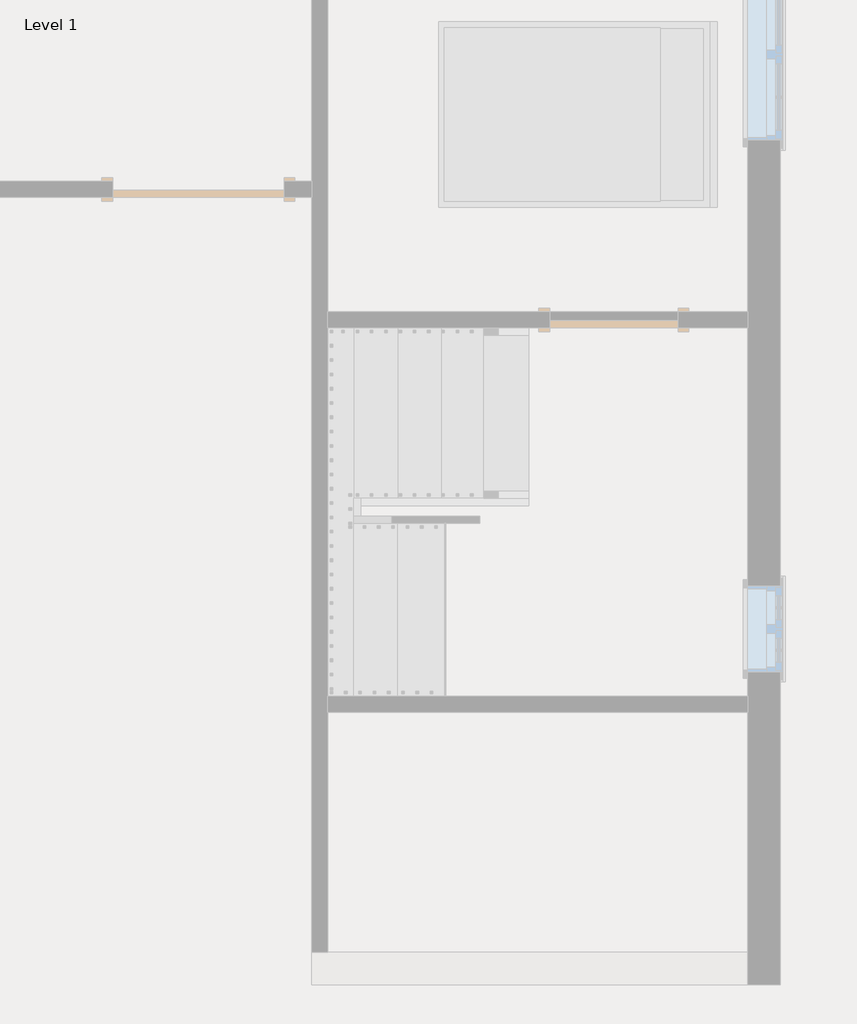
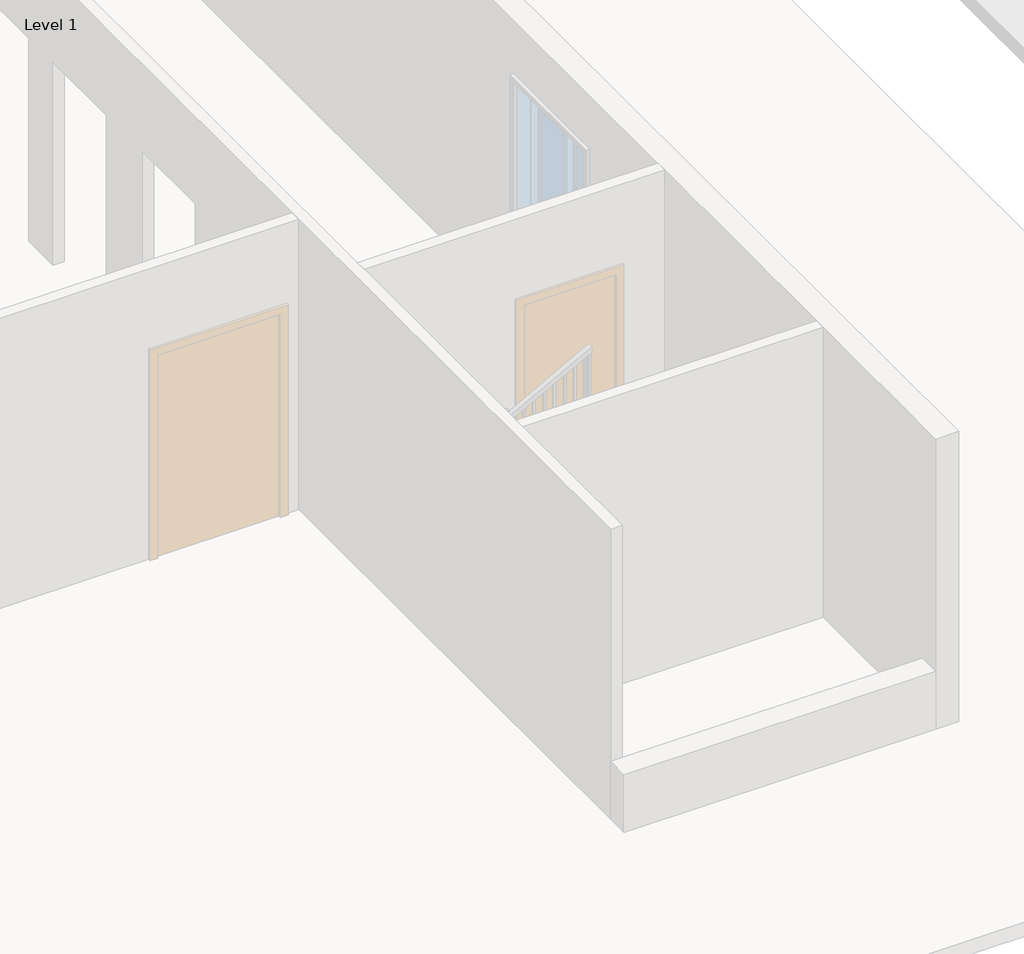
# One storey, part 3 of 7: 2 railings.
"""IFC4 building model written with IfcOpenShell, lengths in millimetres."""

from ifc_helpers import new_model, si_unit, frame, origin, place, context, project, spatial, polyline, outline, extrude, faceted_brep, element, save

model = new_model("IFC4")

# Units and contexts
model_context = context("Model", 3, world=origin())
ifc_project = project(units=[si_unit("LENGTHUNIT", "METRE", prefix="MILLI")], contexts=[model_context])

# Site, building, storey
site = spatial("IfcSite", under=ifc_project)
building = spatial("IfcBuilding", under=site)
storey = spatial("IfcBuildingStorey", under=building, Name="Level 1", Elevation=0.0)

# Railings
placement = place(None, origin())
element("IfcRailing", 1, ObjectType="Handrail - Rectangular", at=placement, inside=storey, context=model_context, shape_type="SolidModel", body=[
    faceted_brep([(7105.1820958, 5435.6, 1083.7333333), (7105.1820958, 5435.6, 1025.8977421), (7105.1820958, 5486.4, 1025.8977421), (7105.1820958, 5486.4, 1083.7333333), (5860.5820958, 5435.6, 1761.0666667), (5847.654197, 5435.6, 1710.2666667), (5847.654197, 5486.4, 1710.2666667), (5860.5820958, 5486.4, 1761.0666667), (5727.7, 5435.6, 1761.0666667), (5727.7, 5435.6, 1710.2666667), (5676.9, 5486.4, 1710.2666667), (5676.9, 5486.4, 1761.0666667), (5727.7, 2997.2, 1761.0666667), (5727.7, 2946.4, 1710.2666667), (5676.9, 2946.4, 1710.2666667), (5676.9, 2997.2, 1761.0666667), (5727.7, 2997.2, 1899.5526009), (5727.7, 2946.4, 1848.7526009), (5676.9, 2946.4, 1848.7526009), (5676.9, 2997.2, 1899.5526009), (5727.7, 2921.0, 1899.5526009), (5727.7, 2921.0, 1848.7526009), (5676.9, 2870.2, 1848.7526009), (5676.9, 2870.2, 1899.5526009), (5803.9, 2921.0, 1899.5526009), (5816.8278988, 2921.0, 1848.7526009), (5816.8278988, 2870.2, 1848.7526009), (5803.9, 2870.2, 1899.5526009), (7105.1820958, 2921.0, 2607.7333333), (7105.1820958, 2870.2, 2607.7333333), (7105.1820958, 2870.2, 2549.8977421), (7105.1820958, 2921.0, 2549.8977421)], [[[0, 1, 2, 3]], [[1, 0, 4, 5]], [[2, 1, 5, 6]], [[3, 2, 6, 7]], [[0, 3, 7, 4]], [[5, 4, 8, 9]], [[6, 5, 9, 10]], [[7, 6, 10, 11]], [[4, 7, 11, 8]], [[9, 8, 12, 13]], [[10, 9, 13, 14]], [[11, 10, 14, 15]], [[8, 11, 15, 12]], [[13, 12, 16, 17]], [[14, 13, 17, 18]], [[15, 14, 18, 19]], [[12, 15, 19, 16]], [[17, 16, 20, 21]], [[18, 17, 21, 22]], [[19, 18, 22, 23]], [[16, 19, 23, 20]], [[21, 20, 24, 25]], [[22, 21, 25, 26]], [[23, 22, 26, 27]], [[20, 23, 27, 24]], [[28, 29, 30, 31]], [[25, 24, 28, 31]], [[26, 25, 31, 30]], [[27, 26, 30, 29]], [[24, 27, 29, 28]]]),
    extrude(outline(polyline([(2510.4108873, 7032.625), (2500.0435403, 7013.575), (1524.0, 7013.575), (1524.0, 7032.625), (2510.4108873, 7032.625)])), frame((0.0, 2886.075, 0.0), z_axis=(0.0, 1.0, 0.0), x_axis=(0.0, 0.0, 1.0)), (0.0, 0.0, 1.0), 19.05),
    extrude(outline(polyline([(2455.1183703, 6931.025), (2444.7510233, 6911.975), (1524.0, 6911.975), (1524.0, 6931.025), (2455.1183703, 6931.025)])), frame((0.0, 2886.075, 0.0), z_axis=(0.0, 1.0, 0.0), x_axis=(0.0, 0.0, 1.0)), (0.0, 0.0, 1.0), 19.05),
    extrude(outline(polyline([(2399.8258533, 6829.425), (2389.4585063, 6810.375), (1524.0, 6810.375), (1524.0, 6829.425), (2399.8258533, 6829.425)])), frame((0.0, 2886.075, 0.0), z_axis=(0.0, 1.0, 0.0), x_axis=(0.0, 0.0, 1.0)), (0.0, 0.0, 1.0), 19.05),
    extrude(outline(polyline([(2344.5333363, 6727.825), (2334.1659893, 6708.775), (1354.6666667, 6708.775), (1354.6666667, 6727.825), (2344.5333363, 6727.825)])), frame((0.0, 2886.075, 0.0), z_axis=(0.0, 1.0, 0.0), x_axis=(0.0, 0.0, 1.0)), (0.0, 0.0, 1.0), 19.05),
    extrude(outline(polyline([(2289.2408192, 6626.225), (2278.8734723, 6607.175), (1354.6666667, 6607.175), (1354.6666667, 6626.225), (2289.2408192, 6626.225)])), frame((0.0, 2886.075, 0.0), z_axis=(0.0, 1.0, 0.0), x_axis=(0.0, 0.0, 1.0)), (0.0, 0.0, 1.0), 19.05),
    extrude(outline(polyline([(2233.9483022, 6524.625), (2223.5809553, 6505.575), (1354.6666667, 6505.575), (1354.6666667, 6524.625), (2233.9483022, 6524.625)])), frame((0.0, 2886.075, 0.0), z_axis=(0.0, 1.0, 0.0), x_axis=(0.0, 0.0, 1.0)), (0.0, 0.0, 1.0), 19.05),
    extrude(outline(polyline([(2178.6557852, 6423.025), (2168.2884383, 6403.975), (1185.3333333, 6403.975), (1185.3333333, 6423.025), (2178.6557852, 6423.025)])), frame((0.0, 2886.075, 0.0), z_axis=(0.0, 1.0, 0.0), x_axis=(0.0, 0.0, 1.0)), (0.0, 0.0, 1.0), 19.05),
    extrude(outline(polyline([(2123.3632682, 6321.425), (2112.9959213, 6302.375), (1185.3333333, 6302.375), (1185.3333333, 6321.425), (2123.3632682, 6321.425)])), frame((0.0, 2886.075, 0.0), z_axis=(0.0, 1.0, 0.0), x_axis=(0.0, 0.0, 1.0)), (0.0, 0.0, 1.0), 19.05),
    extrude(outline(polyline([(2068.0707512, 6219.825), (2057.7034043, 6200.775), (1185.3333333, 6200.775), (1185.3333333, 6219.825), (2068.0707512, 6219.825)])), frame((0.0, 2886.075, 0.0), z_axis=(0.0, 1.0, 0.0), x_axis=(0.0, 0.0, 1.0)), (0.0, 0.0, 1.0), 19.05),
    extrude(outline(polyline([(2012.7782342, 6118.225), (2002.4108873, 6099.175), (1016.0, 6099.175), (1016.0, 6118.225), (2012.7782342, 6118.225)])), frame((0.0, 2886.075, 0.0), z_axis=(0.0, 1.0, 0.0), x_axis=(0.0, 0.0, 1.0)), (0.0, 0.0, 1.0), 19.05),
    extrude(outline(polyline([(1957.4857172, 6016.625), (1947.1183703, 5997.575), (1016.0, 5997.575), (1016.0, 6016.625), (1957.4857172, 6016.625)])), frame((0.0, 2886.075, 0.0), z_axis=(0.0, 1.0, 0.0), x_axis=(0.0, 0.0, 1.0)), (0.0, 0.0, 1.0), 19.05),
    extrude(outline(polyline([(1902.1932002, 5915.025), (1891.8258533, 5895.975), (1016.0, 5895.975), (1016.0, 5915.025), (1902.1932002, 5915.025)])), frame((0.0, 2886.075, 0.0), z_axis=(0.0, 1.0, 0.0), x_axis=(0.0, 0.0, 1.0)), (0.0, 0.0, 1.0), 19.05),
    extrude(outline(polyline([(1846.9006832, 5813.425), (1836.5333363, 5794.375), (846.6666667, 5794.375), (846.6666667, 5813.425), (1846.9006832, 5813.425)])), frame((0.0, 2886.075, 0.0), z_axis=(0.0, 1.0, 0.0), x_axis=(0.0, 0.0, 1.0)), (0.0, 0.0, 1.0), 19.05),
    extrude(outline(polyline([(5692.775, 2930.525), (5711.825, 2930.525), (5711.825, 2911.475), (5692.775, 2911.475), (5692.775, 2930.525)])), frame((0.0, 0.0, 846.6666667), z_axis=(0.0, 0.0, 1.0), x_axis=(1.0, 0.0, 0.0)), (0.0, 0.0, 1.0), 1002.0859343),
    extrude(outline(polyline([(5692.775, 3032.125), (5711.825, 3032.125), (5711.825, 3013.075), (5692.775, 3013.075), (5692.775, 3032.125)])), frame((0.0, 0.0, 846.6666667), z_axis=(0.0, 0.0, 1.0), x_axis=(1.0, 0.0, 0.0)), (0.0, 0.0, 1.0), 863.6),
    extrude(outline(polyline([(5692.775, 3133.725), (5711.825, 3133.725), (5711.825, 3114.675), (5692.775, 3114.675), (5692.775, 3133.725)])), frame((0.0, 0.0, 846.6666667), z_axis=(0.0, 0.0, 1.0), x_axis=(1.0, 0.0, 0.0)), (0.0, 0.0, 1.0), 863.6),
    extrude(outline(polyline([(5692.775, 3235.325), (5711.825, 3235.325), (5711.825, 3216.275), (5692.775, 3216.275), (5692.775, 3235.325)])), frame((0.0, 0.0, 846.6666667), z_axis=(0.0, 0.0, 1.0), x_axis=(1.0, 0.0, 0.0)), (0.0, 0.0, 1.0), 863.6),
    extrude(outline(polyline([(5692.775, 3336.925), (5711.825, 3336.925), (5711.825, 3317.875), (5692.775, 3317.875), (5692.775, 3336.925)])), frame((0.0, 0.0, 846.6666667), z_axis=(0.0, 0.0, 1.0), x_axis=(1.0, 0.0, 0.0)), (0.0, 0.0, 1.0), 863.6),
    extrude(outline(polyline([(5692.775, 3438.525), (5711.825, 3438.525), (5711.825, 3419.475), (5692.775, 3419.475), (5692.775, 3438.525)])), frame((0.0, 0.0, 846.6666667), z_axis=(0.0, 0.0, 1.0), x_axis=(1.0, 0.0, 0.0)), (0.0, 0.0, 1.0), 863.6),
    extrude(outline(polyline([(5692.775, 3540.125), (5711.825, 3540.125), (5711.825, 3521.075), (5692.775, 3521.075), (5692.775, 3540.125)])), frame((0.0, 0.0, 846.6666667), z_axis=(0.0, 0.0, 1.0), x_axis=(1.0, 0.0, 0.0)), (0.0, 0.0, 1.0), 863.6),
    extrude(outline(polyline([(5692.775, 3641.725), (5711.825, 3641.725), (5711.825, 3622.675), (5692.775, 3622.675), (5692.775, 3641.725)])), frame((0.0, 0.0, 846.6666667), z_axis=(0.0, 0.0, 1.0), x_axis=(1.0, 0.0, 0.0)), (0.0, 0.0, 1.0), 863.6),
    extrude(outline(polyline([(5692.775, 3743.325), (5711.825, 3743.325), (5711.825, 3724.275), (5692.775, 3724.275), (5692.775, 3743.325)])), frame((0.0, 0.0, 846.6666667), z_axis=(0.0, 0.0, 1.0), x_axis=(1.0, 0.0, 0.0)), (0.0, 0.0, 1.0), 863.6),
    extrude(outline(polyline([(5692.775, 3844.925), (5711.825, 3844.925), (5711.825, 3825.875), (5692.775, 3825.875), (5692.775, 3844.925)])), frame((0.0, 0.0, 846.6666667), z_axis=(0.0, 0.0, 1.0), x_axis=(1.0, 0.0, 0.0)), (0.0, 0.0, 1.0), 863.6),
    extrude(outline(polyline([(5692.775, 3946.525), (5711.825, 3946.525), (5711.825, 3927.475), (5692.775, 3927.475), (5692.775, 3946.525)])), frame((0.0, 0.0, 846.6666667), z_axis=(0.0, 0.0, 1.0), x_axis=(1.0, 0.0, 0.0)), (0.0, 0.0, 1.0), 863.6),
    extrude(outline(polyline([(5692.775, 4048.125), (5711.825, 4048.125), (5711.825, 4029.075), (5692.775, 4029.075), (5692.775, 4048.125)])), frame((0.0, 0.0, 846.6666667), z_axis=(0.0, 0.0, 1.0), x_axis=(1.0, 0.0, 0.0)), (0.0, 0.0, 1.0), 863.6),
    extrude(outline(polyline([(5692.775, 4149.725), (5711.825, 4149.725), (5711.825, 4130.675), (5692.775, 4130.675), (5692.775, 4149.725)])), frame((0.0, 0.0, 846.6666667), z_axis=(0.0, 0.0, 1.0), x_axis=(1.0, 0.0, 0.0)), (0.0, 0.0, 1.0), 863.6),
    extrude(outline(polyline([(5692.775, 4251.325), (5711.825, 4251.325), (5711.825, 4232.275), (5692.775, 4232.275), (5692.775, 4251.325)])), frame((0.0, 0.0, 846.6666667), z_axis=(0.0, 0.0, 1.0), x_axis=(1.0, 0.0, 0.0)), (0.0, 0.0, 1.0), 863.6),
    extrude(outline(polyline([(5692.775, 4352.925), (5711.825, 4352.925), (5711.825, 4333.875), (5692.775, 4333.875), (5692.775, 4352.925)])), frame((0.0, 0.0, 846.6666667), z_axis=(0.0, 0.0, 1.0), x_axis=(1.0, 0.0, 0.0)), (0.0, 0.0, 1.0), 863.6),
    extrude(outline(polyline([(5692.775, 4454.525), (5711.825, 4454.525), (5711.825, 4435.475), (5692.775, 4435.475), (5692.775, 4454.525)])), frame((0.0, 0.0, 846.6666667), z_axis=(0.0, 0.0, 1.0), x_axis=(1.0, 0.0, 0.0)), (0.0, 0.0, 1.0), 863.6),
    extrude(outline(polyline([(5692.775, 4556.125), (5711.825, 4556.125), (5711.825, 4537.075), (5692.775, 4537.075), (5692.775, 4556.125)])), frame((0.0, 0.0, 846.6666667), z_axis=(0.0, 0.0, 1.0), x_axis=(1.0, 0.0, 0.0)), (0.0, 0.0, 1.0), 863.6),
    extrude(outline(polyline([(5692.775, 4657.725), (5711.825, 4657.725), (5711.825, 4638.675), (5692.775, 4638.675), (5692.775, 4657.725)])), frame((0.0, 0.0, 846.6666667), z_axis=(0.0, 0.0, 1.0), x_axis=(1.0, 0.0, 0.0)), (0.0, 0.0, 1.0), 863.6),
    extrude(outline(polyline([(5692.775, 4759.325), (5711.825, 4759.325), (5711.825, 4740.275), (5692.775, 4740.275), (5692.775, 4759.325)])), frame((0.0, 0.0, 846.6666667), z_axis=(0.0, 0.0, 1.0), x_axis=(1.0, 0.0, 0.0)), (0.0, 0.0, 1.0), 863.6),
    extrude(outline(polyline([(5692.775, 4860.925), (5711.825, 4860.925), (5711.825, 4841.875), (5692.775, 4841.875), (5692.775, 4860.925)])), frame((0.0, 0.0, 846.6666667), z_axis=(0.0, 0.0, 1.0), x_axis=(1.0, 0.0, 0.0)), (0.0, 0.0, 1.0), 863.6),
    extrude(outline(polyline([(5692.775, 4962.525), (5711.825, 4962.525), (5711.825, 4943.475), (5692.775, 4943.475), (5692.775, 4962.525)])), frame((0.0, 0.0, 846.6666667), z_axis=(0.0, 0.0, 1.0), x_axis=(1.0, 0.0, 0.0)), (0.0, 0.0, 1.0), 863.6),
    extrude(outline(polyline([(5692.775, 5064.125), (5711.825, 5064.125), (5711.825, 5045.075), (5692.775, 5045.075), (5692.775, 5064.125)])), frame((0.0, 0.0, 846.6666667), z_axis=(0.0, 0.0, 1.0), x_axis=(1.0, 0.0, 0.0)), (0.0, 0.0, 1.0), 863.6),
    extrude(outline(polyline([(5692.775, 5165.725), (5711.825, 5165.725), (5711.825, 5146.675), (5692.775, 5146.675), (5692.775, 5165.725)])), frame((0.0, 0.0, 846.6666667), z_axis=(0.0, 0.0, 1.0), x_axis=(1.0, 0.0, 0.0)), (0.0, 0.0, 1.0), 863.6),
    extrude(outline(polyline([(5692.775, 5267.325), (5711.825, 5267.325), (5711.825, 5248.275), (5692.775, 5248.275), (5692.775, 5267.325)])), frame((0.0, 0.0, 846.6666667), z_axis=(0.0, 0.0, 1.0), x_axis=(1.0, 0.0, 0.0)), (0.0, 0.0, 1.0), 863.6),
    extrude(outline(polyline([(5692.775, 5368.925), (5711.825, 5368.925), (5711.825, 5349.875), (5692.775, 5349.875), (5692.775, 5368.925)])), frame((0.0, 0.0, 846.6666667), z_axis=(0.0, 0.0, 1.0), x_axis=(1.0, 0.0, 0.0)), (0.0, 0.0, 1.0), 863.6),
    extrude(outline(polyline([(5793.9070958, 5470.525), (5793.9070958, 5451.475), (5774.8570958, 5451.475), (5774.8570958, 5470.525), (5793.9070958, 5470.525)])), frame((0.0, 0.0, 846.6666667), z_axis=(0.0, 0.0, 1.0), x_axis=(1.0, 0.0, 0.0)), (0.0, 0.0, 1.0), 863.6),
    extrude(outline(polyline([(1684.2242727, 5895.5070958), (1694.5916197, 5876.4570958), (677.3333333, 5876.4570958), (677.3333333, 5895.5070958), (1684.2242727, 5895.5070958)])), frame((0.0, 5451.475, 0.0), z_axis=(0.0, 1.0, 0.0), x_axis=(0.0, 0.0, 1.0)), (0.0, 0.0, 1.0), 19.05),
    extrude(outline(polyline([(1628.9317557, 5997.1070958), (1639.2991027, 5978.0570958), (677.3333333, 5978.0570958), (677.3333333, 5997.1070958), (1628.9317557, 5997.1070958)])), frame((0.0, 5451.475, 0.0), z_axis=(0.0, 1.0, 0.0), x_axis=(0.0, 0.0, 1.0)), (0.0, 0.0, 1.0), 19.05),
    extrude(outline(polyline([(1573.6392387, 6098.7070958), (1584.0065857, 6079.6570958), (677.3333333, 6079.6570958), (677.3333333, 6098.7070958), (1573.6392387, 6098.7070958)])), frame((0.0, 5451.475, 0.0), z_axis=(0.0, 1.0, 0.0), x_axis=(0.0, 0.0, 1.0)), (0.0, 0.0, 1.0), 19.05),
    extrude(outline(polyline([(1518.3467217, 6200.3070958), (1528.7140687, 6181.2570958), (508.0, 6181.2570958), (508.0, 6200.3070958), (1518.3467217, 6200.3070958)])), frame((0.0, 5451.475, 0.0), z_axis=(0.0, 1.0, 0.0), x_axis=(0.0, 0.0, 1.0)), (0.0, 0.0, 1.0), 19.05),
    extrude(outline(polyline([(1463.0542047, 6301.9070958), (1473.4215517, 6282.8570958), (508.0, 6282.8570958), (508.0, 6301.9070958), (1463.0542047, 6301.9070958)])), frame((0.0, 5451.475, 0.0), z_axis=(0.0, 1.0, 0.0), x_axis=(0.0, 0.0, 1.0)), (0.0, 0.0, 1.0), 19.05),
    extrude(outline(polyline([(1407.7616877, 6403.5070958), (1418.1290347, 6384.4570958), (508.0, 6384.4570958), (508.0, 6403.5070958), (1407.7616877, 6403.5070958)])), frame((0.0, 5451.475, 0.0), z_axis=(0.0, 1.0, 0.0), x_axis=(0.0, 0.0, 1.0)), (0.0, 0.0, 1.0), 19.05),
    extrude(outline(polyline([(1352.4691707, 6505.1070958), (1362.8365176, 6486.0570958), (338.6666667, 6486.0570958), (338.6666667, 6505.1070958), (1352.4691707, 6505.1070958)])), frame((0.0, 5451.475, 0.0), z_axis=(0.0, 1.0, 0.0), x_axis=(0.0, 0.0, 1.0)), (0.0, 0.0, 1.0), 19.05),
    extrude(outline(polyline([(1297.1766537, 6606.7070958), (1307.5440006, 6587.6570958), (338.6666667, 6587.6570958), (338.6666667, 6606.7070958), (1297.1766537, 6606.7070958)])), frame((0.0, 5451.475, 0.0), z_axis=(0.0, 1.0, 0.0), x_axis=(0.0, 0.0, 1.0)), (0.0, 0.0, 1.0), 19.05),
    extrude(outline(polyline([(1241.8841367, 6708.3070958), (1252.2514836, 6689.2570958), (338.6666667, 6689.2570958), (338.6666667, 6708.3070958), (1241.8841367, 6708.3070958)])), frame((0.0, 5451.475, 0.0), z_axis=(0.0, 1.0, 0.0), x_axis=(0.0, 0.0, 1.0)), (0.0, 0.0, 1.0), 19.05),
    extrude(outline(polyline([(1186.5916197, 6809.9070958), (1196.9589666, 6790.8570958), (169.3333333, 6790.8570958), (169.3333333, 6809.9070958), (1186.5916197, 6809.9070958)])), frame((0.0, 5451.475, 0.0), z_axis=(0.0, 1.0, 0.0), x_axis=(0.0, 0.0, 1.0)), (0.0, 0.0, 1.0), 19.05),
    extrude(outline(polyline([(1131.2991027, 6911.5070958), (1141.6664496, 6892.4570958), (169.3333333, 6892.4570958), (169.3333333, 6911.5070958), (1131.2991027, 6911.5070958)])), frame((0.0, 5451.475, 0.0), z_axis=(0.0, 1.0, 0.0), x_axis=(0.0, 0.0, 1.0)), (0.0, 0.0, 1.0), 19.05),
    extrude(outline(polyline([(1076.0065857, 7013.1070958), (1086.3739326, 6994.0570958), (169.3333333, 6994.0570958), (169.3333333, 7013.1070958), (1076.0065857, 7013.1070958)])), frame((0.0, 5451.475, 0.0), z_axis=(0.0, 1.0, 0.0), x_axis=(0.0, 0.0, 1.0)), (0.0, 0.0, 1.0), 19.05),
    extrude(outline(polyline([(5692.775, 2905.125), (5711.825, 2905.125), (5711.825, 2886.075), (5692.775, 2886.075), (5692.775, 2905.125)])), frame((0.0, 0.0, 846.6666667), z_axis=(0.0, 0.0, 1.0), x_axis=(1.0, 0.0, 0.0)), (0.0, 0.0, 1.0), 1002.0859343),
    extrude(outline(polyline([(5711.825, 5470.525), (5711.825, 5451.475), (5692.775, 5451.475), (5692.775, 5470.525), (5711.825, 5470.525)])), frame((0.0, 0.0, 846.6666667), z_axis=(0.0, 0.0, 1.0), x_axis=(1.0, 0.0, 0.0)), (0.0, 0.0, 1.0), 863.6),
    extrude(outline(polyline([(2549.8977421, 7105.1820958), (2539.5303952, 7086.1320958), (1524.0, 7086.1320958), (1524.0, 7105.1820958), (2549.8977421, 7105.1820958)])), frame((0.0, 2886.075, 0.0), z_axis=(0.0, 1.0, 0.0), x_axis=(0.0, 0.0, 1.0)), (0.0, 0.0, 1.0), 19.05),
    extrude(outline(polyline([(1025.8977421, 7105.1820958), (1036.2650891, 7086.1320958), (169.3333333, 7086.1320958), (169.3333333, 7105.1820958), (1025.8977421, 7105.1820958)])), frame((0.0, 5451.475, 0.0), z_axis=(0.0, 1.0, 0.0), x_axis=(0.0, 0.0, 1.0)), (0.0, 0.0, 1.0), 19.05),
])
element("IfcRailing", 2, ObjectType="Handrail - Rectangular", at=placement, inside=storey, context=model_context, shape_type="SolidModel", body=[
    faceted_brep([(7105.1820958, 4274.6882626, 1083.7333333), (7105.1820958, 4274.6882626, 1025.8977421), (7105.1820958, 4325.4882626, 1025.8977421), (7105.1820958, 4325.4882626, 1083.7333333), (5936.7820958, 4274.6882626, 1719.5972789), (5885.9820958, 4274.6882626, 1689.4079462), (5885.9820958, 4325.4882626, 1689.4079462), (5936.7820958, 4325.4882626, 1719.5972789), (5936.7820958, 4274.6882626, 1761.0666667), (5885.9820958, 4274.6882626, 1710.2666667), (5885.9820958, 4325.4882626, 1710.2666667), (5936.7820958, 4325.4882626, 1761.0666667), (5860.5820958, 4274.6882626, 1761.0666667), (5860.5820958, 4274.6882626, 1710.2666667), (5809.7820958, 4325.4882626, 1710.2666667), (5809.7820958, 4325.4882626, 1761.0666667), (5860.5820958, 4198.4882626, 1761.0666667), (5860.5820958, 4198.4882626, 1710.2666667), (5809.7820958, 4198.4882626, 1710.2666667), (5809.7820958, 4198.4882626, 1761.0666667), (5860.5820958, 4173.0882626, 1761.0666667), (5860.5820958, 4122.2882626, 1710.2666667), (5809.7820958, 4122.2882626, 1710.2666667), (5809.7820958, 4173.0882626, 1761.0666667), (5860.5820958, 4173.0882626, 1971.8693878), (5860.5820958, 4122.2882626, 1921.0693878), (5809.7820958, 4122.2882626, 1921.0693878), (5809.7820958, 4173.0882626, 1971.8693878), (5860.5820958, 4096.8882626, 1971.8693878), (5860.5820958, 4096.8882626, 1921.0693878), (5809.7820958, 4046.0882626, 1921.0693878), (5809.7820958, 4046.0882626, 1971.8693878), (5936.7820958, 4096.8882626, 1971.8693878), (5949.7099946, 4096.8882626, 1921.0693878), (5949.7099946, 4046.0882626, 1921.0693878), (5936.7820958, 4046.0882626, 1971.8693878), (7105.1820958, 4096.8882626, 2607.7333333), (7105.1820958, 4046.0882626, 2607.7333333), (7105.1820958, 4046.0882626, 2549.8977421), (7105.1820958, 4096.8882626, 2549.8977421)], [[[0, 1, 2, 3]], [[1, 0, 4, 5]], [[2, 1, 5, 6]], [[3, 2, 6, 7]], [[0, 3, 7, 4]], [[5, 4, 8, 9]], [[6, 5, 9, 10]], [[7, 6, 10, 11]], [[4, 7, 11, 8]], [[9, 8, 12, 13]], [[10, 9, 13, 14]], [[11, 10, 14, 15]], [[8, 11, 15, 12]], [[13, 12, 16, 17]], [[14, 13, 17, 18]], [[15, 14, 18, 19]], [[12, 15, 19, 16]], [[17, 16, 20, 21]], [[18, 17, 21, 22]], [[19, 18, 22, 23]], [[16, 19, 23, 20]], [[21, 20, 24, 25]], [[22, 21, 25, 26]], [[23, 22, 26, 27]], [[20, 23, 27, 24]], [[25, 24, 28, 29]], [[26, 25, 29, 30]], [[27, 26, 30, 31]], [[24, 27, 31, 28]], [[29, 28, 32, 33]], [[30, 29, 33, 34]], [[31, 30, 34, 35]], [[28, 31, 35, 32]], [[36, 37, 38, 39]], [[33, 32, 36, 39]], [[34, 33, 39, 38]], [[35, 34, 38, 37]], [[32, 35, 37, 36]]]),
    extrude(outline(polyline([(2517.0678102, 7044.8570958), (1524.0, 7044.8570958), (1524.0, 7063.9070958), (2527.4351571, 7063.9070958), (2517.0678102, 7044.8570958)])), frame((0.0, 4061.9632626, 0.0), z_axis=(0.0, 1.0, 0.0), x_axis=(0.0, 0.0, 1.0)), (0.0, 0.0, 1.0), 19.05),
    extrude(outline(polyline([(2461.7752932, 6943.2570958), (1524.0, 6943.2570958), (1524.0, 6962.3070958), (2472.1426401, 6962.3070958), (2461.7752932, 6943.2570958)])), frame((0.0, 4061.9632626, 0.0), z_axis=(0.0, 1.0, 0.0), x_axis=(0.0, 0.0, 1.0)), (0.0, 0.0, 1.0), 19.05),
    extrude(outline(polyline([(2406.4827761, 6841.6570958), (1524.0, 6841.6570958), (1524.0, 6860.7070958), (2416.8501231, 6860.7070958), (2406.4827761, 6841.6570958)])), frame((0.0, 4061.9632626, 0.0), z_axis=(0.0, 1.0, 0.0), x_axis=(0.0, 0.0, 1.0)), (0.0, 0.0, 1.0), 19.05),
    extrude(outline(polyline([(2351.1902591, 6740.0570958), (1354.6666667, 6740.0570958), (1354.6666667, 6759.1070958), (2361.5576061, 6759.1070958), (2351.1902591, 6740.0570958)])), frame((0.0, 4061.9632626, 0.0), z_axis=(0.0, 1.0, 0.0), x_axis=(0.0, 0.0, 1.0)), (0.0, 0.0, 1.0), 19.05),
    extrude(outline(polyline([(2295.8977421, 6638.4570958), (1354.6666667, 6638.4570958), (1354.6666667, 6657.5070958), (2306.2650891, 6657.5070958), (2295.8977421, 6638.4570958)])), frame((0.0, 4061.9632626, 0.0), z_axis=(0.0, 1.0, 0.0), x_axis=(0.0, 0.0, 1.0)), (0.0, 0.0, 1.0), 19.05),
    extrude(outline(polyline([(2240.6052251, 6536.8570958), (1354.6666667, 6536.8570958), (1354.6666667, 6555.9070958), (2250.9725721, 6555.9070958), (2240.6052251, 6536.8570958)])), frame((0.0, 4061.9632626, 0.0), z_axis=(0.0, 1.0, 0.0), x_axis=(0.0, 0.0, 1.0)), (0.0, 0.0, 1.0), 19.05),
    extrude(outline(polyline([(2185.3127081, 6435.2570958), (1185.3333333, 6435.2570958), (1185.3333333, 6454.3070958), (2195.6800551, 6454.3070958), (2185.3127081, 6435.2570958)])), frame((0.0, 4061.9632626, 0.0), z_axis=(0.0, 1.0, 0.0), x_axis=(0.0, 0.0, 1.0)), (0.0, 0.0, 1.0), 19.05),
    extrude(outline(polyline([(2130.0201911, 6333.6570958), (1185.3333333, 6333.6570958), (1185.3333333, 6352.7070958), (2140.3875381, 6352.7070958), (2130.0201911, 6333.6570958)])), frame((0.0, 4061.9632626, 0.0), z_axis=(0.0, 1.0, 0.0), x_axis=(0.0, 0.0, 1.0)), (0.0, 0.0, 1.0), 19.05),
    extrude(outline(polyline([(2074.7276741, 6232.0570958), (1185.3333333, 6232.0570958), (1185.3333333, 6251.1070958), (2085.095021, 6251.1070958), (2074.7276741, 6232.0570958)])), frame((0.0, 4061.9632626, 0.0), z_axis=(0.0, 1.0, 0.0), x_axis=(0.0, 0.0, 1.0)), (0.0, 0.0, 1.0), 19.05),
    extrude(outline(polyline([(2019.4351571, 6130.4570958), (1016.0, 6130.4570958), (1016.0, 6149.5070958), (2029.802504, 6149.5070958), (2019.4351571, 6130.4570958)])), frame((0.0, 4061.9632626, 0.0), z_axis=(0.0, 1.0, 0.0), x_axis=(0.0, 0.0, 1.0)), (0.0, 0.0, 1.0), 19.05),
    extrude(outline(polyline([(1964.1426401, 6028.8570958), (1016.0, 6028.8570958), (1016.0, 6047.9070958), (1974.509987, 6047.9070958), (1964.1426401, 6028.8570958)])), frame((0.0, 4061.9632626, 0.0), z_axis=(0.0, 1.0, 0.0), x_axis=(0.0, 0.0, 1.0)), (0.0, 0.0, 1.0), 19.05),
    extrude(outline(polyline([(1908.8501231, 5927.2570958), (1016.0, 5927.2570958), (1016.0, 5946.3070958), (1919.21747, 5946.3070958), (1908.8501231, 5927.2570958)])), frame((0.0, 4061.9632626, 0.0), z_axis=(0.0, 1.0, 0.0), x_axis=(0.0, 0.0, 1.0)), (0.0, 0.0, 1.0), 19.05),
    extrude(outline(polyline([(5844.7070958, 4106.4132626), (5844.7070958, 4087.3632626), (5825.6570958, 4087.3632626), (5825.6570958, 4106.4132626), (5844.7070958, 4106.4132626)])), frame((0.0, 0.0, 846.6666667), z_axis=(0.0, 0.0, 1.0), x_axis=(1.0, 0.0, 0.0)), (0.0, 0.0, 1.0), 1074.4027211),
    extrude(outline(polyline([(5844.7070958, 4208.0132626), (5844.7070958, 4188.9632626), (5825.6570958, 4188.9632626), (5825.6570958, 4208.0132626), (5844.7070958, 4208.0132626)])), frame((0.0, 0.0, 846.6666667), z_axis=(0.0, 0.0, 1.0), x_axis=(1.0, 0.0, 0.0)), (0.0, 0.0, 1.0), 863.6),
    extrude(outline(polyline([(5895.5070958, 4290.5632626), (5876.4570958, 4290.5632626), (5876.4570958, 4309.6132626), (5895.5070958, 4309.6132626), (5895.5070958, 4290.5632626)])), frame((0.0, 0.0, 677.3333333), z_axis=(0.0, 0.0, 1.0), x_axis=(1.0, 0.0, 0.0)), (0.0, 0.0, 1.0), 1032.9333333),
    extrude(outline(polyline([(1639.2991027, 5978.0570958), (677.3333333, 5978.0570958), (677.3333333, 5997.1070958), (1628.9317557, 5997.1070958), (1639.2991027, 5978.0570958)])), frame((0.0, 4290.5632626, 0.0), z_axis=(0.0, 1.0, 0.0), x_axis=(0.0, 0.0, 1.0)), (0.0, 0.0, 1.0), 19.05),
    extrude(outline(polyline([(1584.0065857, 6079.6570958), (677.3333333, 6079.6570958), (677.3333333, 6098.7070958), (1573.6392387, 6098.7070958), (1584.0065857, 6079.6570958)])), frame((0.0, 4290.5632626, 0.0), z_axis=(0.0, 1.0, 0.0), x_axis=(0.0, 0.0, 1.0)), (0.0, 0.0, 1.0), 19.05),
    extrude(outline(polyline([(1528.7140687, 6181.2570958), (508.0, 6181.2570958), (508.0, 6200.3070958), (1518.3467217, 6200.3070958), (1528.7140687, 6181.2570958)])), frame((0.0, 4290.5632626, 0.0), z_axis=(0.0, 1.0, 0.0), x_axis=(0.0, 0.0, 1.0)), (0.0, 0.0, 1.0), 19.05),
    extrude(outline(polyline([(1473.4215517, 6282.8570958), (508.0, 6282.8570958), (508.0, 6301.9070958), (1463.0542047, 6301.9070958), (1473.4215517, 6282.8570958)])), frame((0.0, 4290.5632626, 0.0), z_axis=(0.0, 1.0, 0.0), x_axis=(0.0, 0.0, 1.0)), (0.0, 0.0, 1.0), 19.05),
    extrude(outline(polyline([(1418.1290347, 6384.4570958), (508.0, 6384.4570958), (508.0, 6403.5070958), (1407.7616877, 6403.5070958), (1418.1290347, 6384.4570958)])), frame((0.0, 4290.5632626, 0.0), z_axis=(0.0, 1.0, 0.0), x_axis=(0.0, 0.0, 1.0)), (0.0, 0.0, 1.0), 19.05),
    extrude(outline(polyline([(1362.8365176, 6486.0570958), (338.6666667, 6486.0570958), (338.6666667, 6505.1070958), (1352.4691707, 6505.1070958), (1362.8365176, 6486.0570958)])), frame((0.0, 4290.5632626, 0.0), z_axis=(0.0, 1.0, 0.0), x_axis=(0.0, 0.0, 1.0)), (0.0, 0.0, 1.0), 19.05),
    extrude(outline(polyline([(1307.5440006, 6587.6570958), (338.6666667, 6587.6570958), (338.6666667, 6606.7070958), (1297.1766537, 6606.7070958), (1307.5440006, 6587.6570958)])), frame((0.0, 4290.5632626, 0.0), z_axis=(0.0, 1.0, 0.0), x_axis=(0.0, 0.0, 1.0)), (0.0, 0.0, 1.0), 19.05),
    extrude(outline(polyline([(1252.2514836, 6689.2570958), (338.6666667, 6689.2570958), (338.6666667, 6708.3070958), (1241.8841367, 6708.3070958), (1252.2514836, 6689.2570958)])), frame((0.0, 4290.5632626, 0.0), z_axis=(0.0, 1.0, 0.0), x_axis=(0.0, 0.0, 1.0)), (0.0, 0.0, 1.0), 19.05),
    extrude(outline(polyline([(1196.9589666, 6790.8570958), (169.3333333, 6790.8570958), (169.3333333, 6809.9070958), (1186.5916197, 6809.9070958), (1196.9589666, 6790.8570958)])), frame((0.0, 4290.5632626, 0.0), z_axis=(0.0, 1.0, 0.0), x_axis=(0.0, 0.0, 1.0)), (0.0, 0.0, 1.0), 19.05),
    extrude(outline(polyline([(1141.6664496, 6892.4570958), (169.3333333, 6892.4570958), (169.3333333, 6911.5070958), (1131.2991027, 6911.5070958), (1141.6664496, 6892.4570958)])), frame((0.0, 4290.5632626, 0.0), z_axis=(0.0, 1.0, 0.0), x_axis=(0.0, 0.0, 1.0)), (0.0, 0.0, 1.0), 19.05),
    extrude(outline(polyline([(1086.3739326, 6994.0570958), (169.3333333, 6994.0570958), (169.3333333, 7013.1070958), (1076.0065857, 7013.1070958), (1086.3739326, 6994.0570958)])), frame((0.0, 4290.5632626, 0.0), z_axis=(0.0, 1.0, 0.0), x_axis=(0.0, 0.0, 1.0)), (0.0, 0.0, 1.0), 19.05),
    extrude(outline(polyline([(5844.7070958, 4081.0132626), (5844.7070958, 4061.9632626), (5825.6570958, 4061.9632626), (5825.6570958, 4081.0132626), (5844.7070958, 4081.0132626)])), frame((0.0, 0.0, 846.6666667), z_axis=(0.0, 0.0, 1.0), x_axis=(1.0, 0.0, 0.0)), (0.0, 0.0, 1.0), 1074.4027211),
    extrude(outline(polyline([(5844.7070958, 4290.5632626), (5825.6570958, 4290.5632626), (5825.6570958, 4309.6132626), (5844.7070958, 4309.6132626), (5844.7070958, 4290.5632626)])), frame((0.0, 0.0, 846.6666667), z_axis=(0.0, 0.0, 1.0), x_axis=(1.0, 0.0, 0.0)), (0.0, 0.0, 1.0), 863.6),
    extrude(outline(polyline([(2539.5303952, 7086.1320958), (1524.0, 7086.1320958), (1524.0, 7105.1820958), (2549.8977421, 7105.1820958), (2539.5303952, 7086.1320958)])), frame((0.0, 4061.9632626, 0.0), z_axis=(0.0, 1.0, 0.0), x_axis=(0.0, 0.0, 1.0)), (0.0, 0.0, 1.0), 19.05),
    extrude(outline(polyline([(1036.2650891, 7086.1320958), (169.3333333, 7086.1320958), (169.3333333, 7105.1820958), (1025.8977421, 7105.1820958), (1036.2650891, 7086.1320958)])), frame((0.0, 4290.5632626, 0.0), z_axis=(0.0, 1.0, 0.0), x_axis=(0.0, 0.0, 1.0)), (0.0, 0.0, 1.0), 19.05),
])

save(model, "model.ifc")

# Revit data of these elements
# Type "Handrail - Rectangular"
#   Assembly Code = "C2010400"
#   built-in parameter 1008612 = 0.0416667 (stored number, unit not read)
#   built-in parameter 1008611 = 0.0416667 (stored number, unit not read)
#   built-in parameter 1008609 = 0.333333 (stored number, unit not read)
#   built-in parameter 1008604 = 0.166667 (stored number, unit not read)
#   built-in parameter 1008603 = 0.166667 (stored number, unit not read)
#   Railing Height = 3' - 0"
#   built-in parameter 1008630 = 2
#   built-in parameter 1008610 = 2
#   built-in parameter 1008618 = Baluster - Square : 3/4"
# Elements 1, 2 (IfcRailing, "Handrail - Rectangular")
#   Phase Created = New Construction
